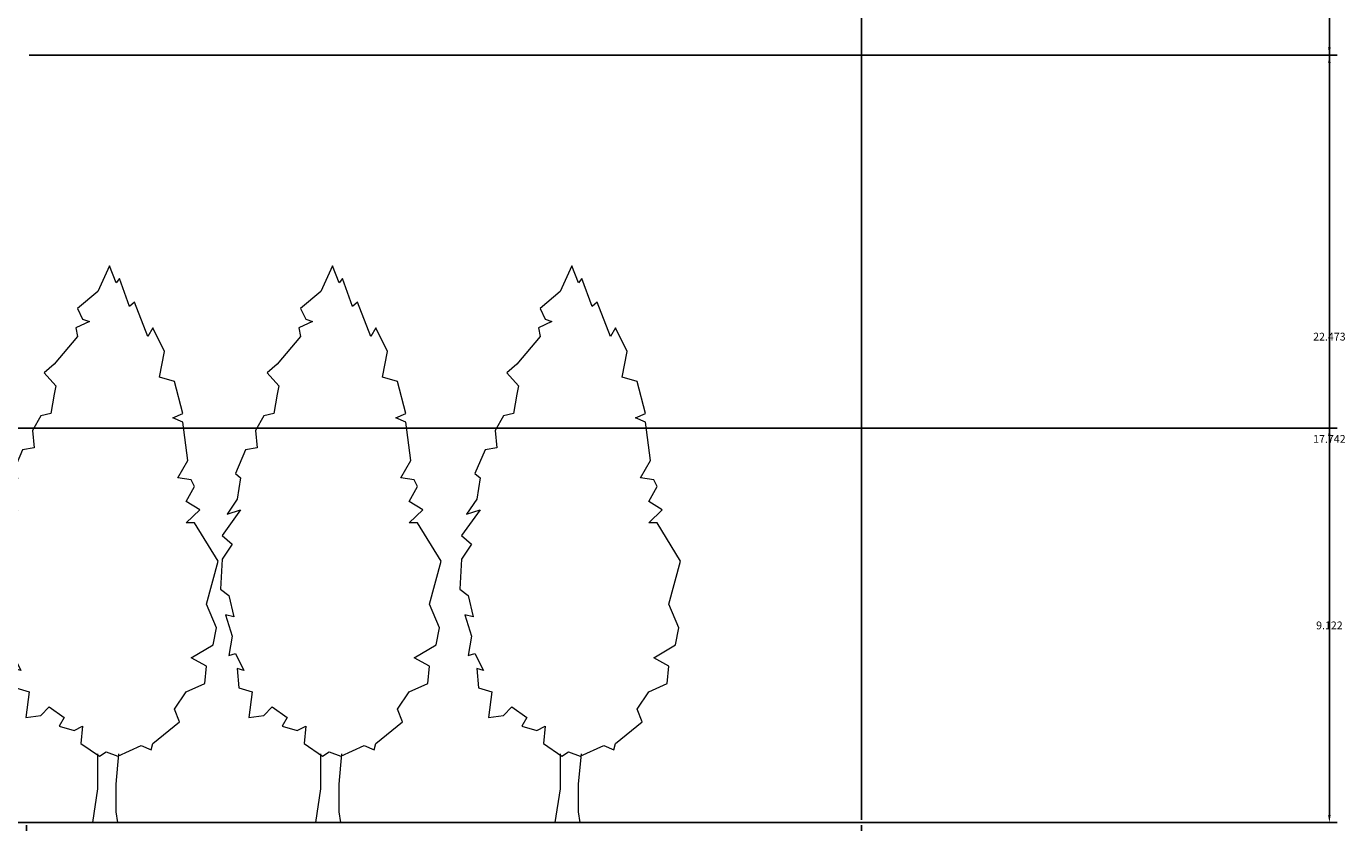
# Model space of a CAD drawing. Units: inches. Extents: x -117 to 121, y -77 to 40.
# Tile 39 of 45: x 91 to 121, y -61 to -43. Entities that reach past the tile are written whole.
import ezdxf

# ---------------------------------------------------------------- set-up
doc = ezdxf.new("R2010")
doc.units = ezdxf.units.IN
doc.header["$MEASUREMENT"] = 0
doc.layers.add('A-ANNO-DIMS', color=2, linetype='Continuous', lineweight=18)
doc.layers.add('L-PLNT', color=3, linetype='Continuous', lineweight=13)
doc.styles.get("Standard").update_dxf_attribs({"font": 'arial.ttf'})
doc.dimstyles.get("Standard").update_dxf_attribs({"dimtxt": 0.18, "dimasz": 0.18, "dimexe": 0.18, "dimexo": 0.0625, "dimgap": 0.09, "dimtad": 0, "dimtih": 1, "dimtoh": 1, "dimdec": 4, "dimzin": 0, "dimdsep": 46, "dimtxsty": 'Standard', "dimcen": 0.09, "dimadec": 0, "dimazin": 0, "dimtfac": 1, "dimtdec": 4, "dimtofl": 0, "dimtmove": 0, "dimatfit": 3, "dimfxl": 1, "dimtolj": 1, "dimtzin": 0, "dimarcsym": 0})

# ---------------------------------------------------------------- blocks, each defined once
blk = doc.blocks.new('*U2')
blk.add_lwpolyline([(-2.754, 191.699), (-6.78, 182.851), (-13.682, 176.953), (-11.956, 173.266), (-9.656, 172.529), (-14.257, 170.317), (-13.682, 167.368), (-21.733, 157.783), (-25.184, 154.834), (-21.158, 150.41), (-21.733, 147.461), (-22.884, 140.825), (-26.334, 140.087), (-29.21, 134.926), (-28.635, 129.028), (-32.661, 128.291), (-36.111, 120.18), (-34.386, 118.706), (-35.536, 111.333), (-38.987, 106.171), (-34.386, 107.646), (-40.712, 98.798), (-37.261, 95.849), (-40.712, 90.688), (-41.287, 80.366), (-38.412, 78.154), (-36.686, 70.781), (-39.562, 71.518), (-37.261, 64.145), (-38.412, 57.509), (-36.111, 58.247), (-33.236, 52.348), (-35.536, 53.086), (-34.961, 46.45), (-30.36, 44.975), (-31.51, 36.128), (-26.334, 36.865), (-23.459, 39.814), (-18.283, 36.128), (-20.008, 33.178), (-14.832, 31.704), (-11.956, 33.178), (-12.531, 27.28), (-6.205, 22.856), (-3.905, 24.331), (0.121, 22.856), (8.173, 26.543), (11.624, 25.068), (12.199, 27.28), (21.4, 34.653), (19.675, 39.077), (23.701, 44.975), (30.027, 47.924), (30.602, 53.823), (25.426, 56.772), (32.903, 61.196), (34.053, 67.094), (30.602, 75.205), (34.628, 89.951), (26.576, 103.222), (23.701, 103.222), (28.302, 107.646), (23.701, 110.595), (26.576, 115.756), (25.426, 117.968), (20.825, 118.706), (24.276, 124.604), (22.551, 137.876), (19.1, 139.35), (22.551, 140.825), (19.675, 151.884), (14.499, 153.359), (16.224, 162.207), (12.199, 170.317), (10.473, 167.368), (5.872, 179.165), (4.147, 177.69), (0.696, 187.275), (-0.454, 185.8)], close=True)
for points in [[(-6.813, 23.669), (-6.813, 11.669), (-8.627, 0)], [(0.387, 23.669), (-0.576, 13.271), (-0.576, 3.686), (0, 0)]]:
    blk.add_lwpolyline(points)
blk = doc.blocks.new('*D7')
at = {"layer": 'A-ANNO-DIMS', "color": 0, "lineweight": -2, "transparency": 16777216}
for p, q in [((-77.763, -61.431), (-77.763, -77.193)), ((90.549, -61.438), (90.549, -77.193)), ((-77.583, -77.013), (6.008, -77.013)), ((90.369, -77.013), (6.778, -77.013))]:
    blk.add_line(p, q, dxfattribs=at)
at = {"layer": 'A-ANNO-DIMS', "color": 0, "transparency": 16777216}
for points in [[(-77.583, -76.983), (-77.583, -77.043), (-77.763, -77.013)], [(90.369, -76.983), (90.369, -77.043), (90.549, -77.013)]]:
    blk.add_solid(points, dxfattribs=at)
at = {"layer": 'Defpoints', "color": 0, "transparency": 16777216}
for p in [(-77.763, -61.369), (90.549, -61.376), (90.549, -77.013)]:
    blk.add_point(p, dxfattribs=at)
at = {"layer": 'A-ANNO-DIMS', "color": 0, "transparency": 16777216, "insert": (6.393, -77.013), "char_height": 0.18, "attachment_point": 5}
blk.add_mtext('\\A1;168.3', dxfattribs=at)
blk = doc.blocks.new('*D8')
at = {"layer": 'A-ANNO-DIMS', "color": 0, "lineweight": -2, "transparency": 16777216}
for p, q in [((90.549, -61.438), (90.549, -77.193)), ((109.85, -61.438), (109.85, -77.193)), ((90.729, -77.013), (99.884, -77.013)), ((109.67, -77.013), (100.515, -77.013))]:
    blk.add_line(p, q, dxfattribs=at)
at = {"layer": 'A-ANNO-DIMS', "color": 0, "transparency": 16777216}
for points in [[(90.729, -76.983), (90.729, -77.043), (90.549, -77.013)], [(109.67, -76.983), (109.67, -77.043), (109.85, -77.013)]]:
    blk.add_solid(points, dxfattribs=at)
at = {"layer": 'Defpoints', "color": 0, "transparency": 16777216}
for p in [(90.549, -61.376), (109.85, -61.376), (109.85, -77.013)]:
    blk.add_point(p, dxfattribs=at)
at = {"layer": 'A-ANNO-DIMS', "color": 0, "transparency": 16777216, "insert": (100.199, -77.013), "char_height": 0.18, "attachment_point": 5}
blk.add_mtext('\\A1;19.3', dxfattribs=at)
blk = doc.blocks.new('*D14')
at = {"layer": 'A-ANNO-DIMS', "color": 0, "lineweight": -2, "transparency": 16777216}
for p, q in [((90.611, -38.902), (120.84, -38.902)), ((120.66, -39.082), (120.66, -49.957)), ((120.66, -61.196), (120.66, -50.321)), ((109.913, -61.376), (120.84, -61.376))]:
    blk.add_line(p, q, dxfattribs=at)
at = {"layer": 'A-ANNO-DIMS', "color": 0, "transparency": 16777216}
for points in [[(120.63, -39.082), (120.69, -39.082), (120.66, -38.902)], [(120.63, -61.196), (120.69, -61.196), (120.66, -61.376)]]:
    blk.add_solid(points, dxfattribs=at)
at = {"layer": 'Defpoints', "color": 0, "transparency": 16777216}
for p in [(90.549, -38.902), (109.85, -61.376), (120.66, -61.376)]:
    blk.add_point(p, dxfattribs=at)
at = {"layer": 'A-ANNO-DIMS', "color": 0, "transparency": 16777216, "insert": (120.66, -50.139), "char_height": 0.18, "attachment_point": 5}
blk.add_mtext('\\A1;22.473', dxfattribs=at)
blk = doc.blocks.new('*D24')
at = {"layer": 'A-ANNO-DIMS', "color": 0, "lineweight": -2, "transparency": 16777216}
for p, q in [((87.242, 3.166), (87.242, 38.61)), ((87.422, 38.43), (98.081, 38.43)), ((109.67, 38.43), (99.011, 38.43)), ((109.85, -61.313), (109.85, 38.61))]:
    blk.add_line(p, q, dxfattribs=at)
at = {"layer": 'A-ANNO-DIMS', "color": 0, "transparency": 16777216}
for points in [[(87.422, 38.46), (87.422, 38.4), (87.242, 38.43)], [(109.67, 38.46), (109.67, 38.4), (109.85, 38.43)]]:
    blk.add_solid(points, dxfattribs=at)
at = {"layer": 'Defpoints', "color": 0, "transparency": 16777216}
for p in [(109.85, 38.43), (87.242, 3.104), (109.85, -61.376)]:
    blk.add_point(p, dxfattribs=at)
at = {"layer": 'A-ANNO-DIMS', "color": 0, "transparency": 16777216, "insert": (98.546, 38.43), "char_height": 0.18, "attachment_point": 5}
blk.add_mtext('\\A1;22.609', dxfattribs=at)
blk = doc.blocks.new('*D31')
at = {"layer": 'A-ANNO-DIMS', "color": 0, "lineweight": -2, "transparency": 16777216}
for p, q in [((87.459, -61.438), (87.459, -77.193)), ((90.549, -61.438), (90.549, -77.193)), ((87.639, -77.013), (88.61, -77.013)), ((90.369, -77.013), (89.397, -77.013))]:
    blk.add_line(p, q, dxfattribs=at)
at = {"layer": 'A-ANNO-DIMS', "color": 0, "transparency": 16777216}
for points in [[(87.639, -76.983), (87.639, -77.043), (87.459, -77.013)], [(90.369, -76.983), (90.369, -77.043), (90.549, -77.013)]]:
    blk.add_solid(points, dxfattribs=at)
at = {"layer": 'Defpoints', "color": 0, "transparency": 16777216}
for p in [(87.459, -61.376), (90.549, -61.376), (90.549, -77.013)]:
    blk.add_point(p, dxfattribs=at)
at = {"layer": 'A-ANNO-DIMS', "color": 0, "transparency": 16777216, "insert": (89.004, -77.013), "char_height": 0.18, "attachment_point": 5}
blk.add_mtext('\\A1;3.090', dxfattribs=at)
blk = doc.blocks.new('*D34')
at = {"layer": 'A-ANNO-DIMS', "color": 0, "lineweight": -2, "transparency": 16777216}
for p, q in [((90.611, -43.633), (120.84, -43.633)), ((120.66, -43.813), (120.66, -52.324)), ((120.66, -61.196), (120.66, -52.685)), ((90.611, -61.376), (120.84, -61.376))]:
    blk.add_line(p, q, dxfattribs=at)
at = {"layer": 'A-ANNO-DIMS', "color": 0, "transparency": 16777216}
for points in [[(120.63, -43.813), (120.69, -43.813), (120.66, -43.633)], [(120.63, -61.196), (120.69, -61.196), (120.66, -61.376)]]:
    blk.add_solid(points, dxfattribs=at)
at = {"layer": 'Defpoints', "color": 0, "transparency": 16777216}
for p in [(90.549, -43.633), (120.66, -43.633), (90.549, -61.376)]:
    blk.add_point(p, dxfattribs=at)
at = {"layer": 'A-ANNO-DIMS', "color": 0, "transparency": 16777216, "insert": (120.66, -52.504), "char_height": 0.18, "attachment_point": 5}
blk.add_mtext('\\A1;17.742', dxfattribs=at)
blk = doc.blocks.new('*D35')
at = {"layer": 'A-ANNO-DIMS', "color": 0, "lineweight": -2, "transparency": 16777216}
for p, q in [((90.611, -41.705), (120.84, -41.705)), ((120.66, -41.885), (120.66, -42.487)), ((120.66, -43.453), (120.66, -42.851)), ((90.611, -43.633), (120.84, -43.633))]:
    blk.add_line(p, q, dxfattribs=at)
at = {"layer": 'A-ANNO-DIMS', "color": 0, "transparency": 16777216}
for points in [[(120.63, -41.885), (120.69, -41.885), (120.66, -41.705)], [(120.63, -43.453), (120.69, -43.453), (120.66, -43.633)]]:
    blk.add_solid(points, dxfattribs=at)
at = {"layer": 'Defpoints', "color": 0, "transparency": 16777216}
for p in [(90.549, -41.705), (120.66, -41.705), (90.549, -43.633)]:
    blk.add_point(p, dxfattribs=at)
at = {"layer": 'A-ANNO-DIMS', "color": 0, "transparency": 16777216, "insert": (120.66, -42.669), "char_height": 0.18, "attachment_point": 5}
blk.add_mtext('\\A1;1.928', dxfattribs=at)
blk = doc.blocks.new('*D38')
at = {"layer": 'A-ANNO-DIMS', "color": 0, "lineweight": -2, "transparency": 16777216}
for p, q in [((87.521, -52.254), (120.84, -52.254)), ((120.66, -52.434), (120.66, -56.633)), ((120.66, -61.196), (120.66, -56.997)), ((87.521, -61.376), (120.84, -61.376))]:
    blk.add_line(p, q, dxfattribs=at)
at = {"layer": 'A-ANNO-DIMS', "color": 0, "transparency": 16777216}
for points in [[(120.63, -52.434), (120.69, -52.434), (120.66, -52.254)], [(120.63, -61.196), (120.69, -61.196), (120.66, -61.376)]]:
    blk.add_solid(points, dxfattribs=at)
at = {"layer": 'Defpoints', "color": 0, "transparency": 16777216}
for p in [(87.459, -52.254), (87.459, -61.376), (120.66, -61.376)]:
    blk.add_point(p, dxfattribs=at)
at = {"layer": 'A-ANNO-DIMS', "color": 0, "transparency": 16777216, "insert": (120.66, -56.815), "char_height": 0.18, "attachment_point": 5}
blk.add_mtext('\\A1;9.122', dxfattribs=at)

msp = doc.modelspace()

# ---------------------------------------------------------------- block references
at = {"layer": 'L-PLNT', "xscale": 0.0671647796176818, "yscale": 0.0671647796176818, "zscale": 0.0671647796176818}
for p in [(92.6522, -61.3752), (97.8058, -61.3752), (103.3411, -61.3752)]:
    msp.add_blockref('*U2', p, dxfattribs=at)

# ---------------------------------------------------------------- dimensions: what is measured, and where the dimension line sits
at = {"layer": 'A-ANNO-DIMS'}
for base, p1, p2, override, picture, middle in [((109.8502, 38.4297), (87.2416, 3.1036), (109.8502, -61.3756), {"dimdec": 3, "dimlfac": 1, "dimrnd": 0, "dimzin": 0, "dimdsep": 46, "dimlunit": 2}, '*D24', (98.5459, 38.4297)), ((90.5486, -77.0135), (-77.7631, -61.3689), (90.5486, -61.3756), {"dimdec": 1, "dimlfac": 1, "dimrnd": 0, "dimzin": 0, "dimdsep": 46, "dimlunit": 2}, '*D7', (6.3928, -77.0135)), ((90.5486, -77.0135), (87.4587, -61.3756), (90.5486, -61.3756), {"dimdec": 3, "dimlfac": 1, "dimrnd": 0, "dimzin": 0, "dimdsep": 46, "dimlunit": 2}, '*D31', (89.0036, -77.0135)), ((109.8502, -77.0135), (90.5486, -61.3756), (109.8502, -61.3756), {"dimdec": 1, "dimlfac": 1, "dimrnd": 0, "dimzin": 0, "dimdsep": 46, "dimlunit": 2}, '*D8', (100.1994, -77.0135))]:
    dim = msp.add_linear_dim(base=base, p1=p1, p2=p2, dimstyle='Standard', override=override, dxfattribs=at)
    dim.commit()
    dim.dimension.update_dxf_attribs({"geometry": picture, "text_midpoint": middle})
for base, p1, p2, picture, middle in [((120.6602, -61.3756), (90.5486, -38.9022), (109.8502, -61.3756), '*D14', (120.6602, -50.1389)), ((120.6602, -41.7053), (90.5486, -43.6334), (90.5486, -41.7053), '*D35', (120.6602, -42.6693)), ((120.6602, -43.6334), (90.5486, -61.3756), (90.5486, -43.6334), '*D34', (120.6602, -52.5045)), ((120.6602, -61.3756), (87.4587, -52.2539), (87.4587, -61.3756), '*D38', (120.6602, -56.8148))]:
    dim = msp.add_linear_dim(base=base, p1=p1, p2=p2, angle=90, dimstyle='Standard', override={"dimdec": 3, "dimlfac": 1, "dimrnd": 0, "dimzin": 0, "dimdsep": 46, "dimlunit": 2}, dxfattribs=at)
    dim.commit()
    dim.dimension.update_dxf_attribs({"geometry": picture, "text_midpoint": middle})

doc.saveas('drawing.dxf')
